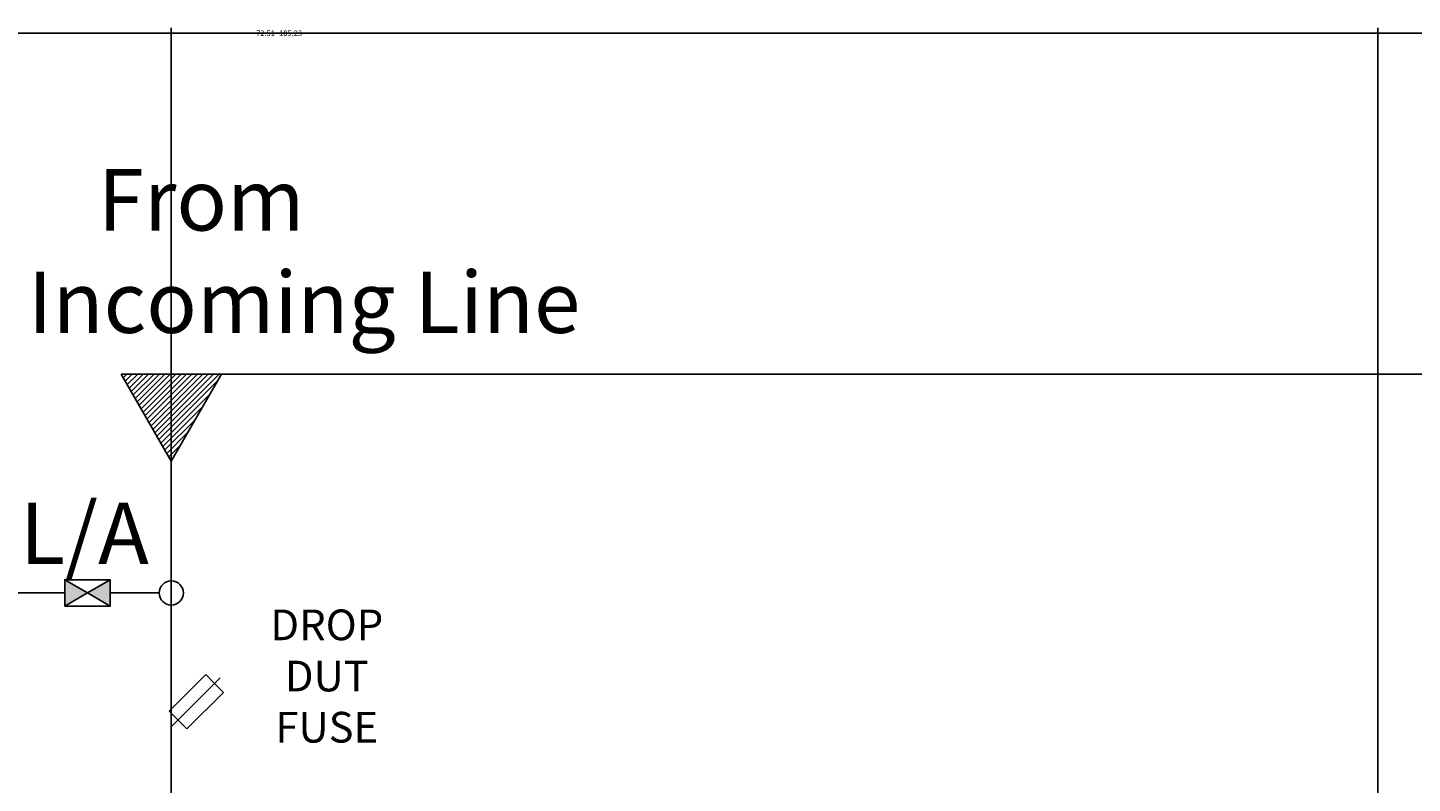
# Model space of a CAD drawing. Units: inches. Extents: x 412 to 584, y 208 to 437.
# Tile 27 of 28: x 495 to 540, y 413 to 437. Entities that reach past the tile are written whole.
import ezdxf

# ---------------------------------------------------------------- set-up
doc = ezdxf.new("R2010")
doc.units = ezdxf.units.IN
doc.header["$MEASUREMENT"] = 0
for name, color, linetype, lineweight in [('A-ANNO-DIMS', 2, 'Continuous', 18), ('E-ANNO-TEXT', 7, 'Continuous', 18), ('E-POWR-EQPM', 3, 'Continuous', 25), ('E-POWR-PATT', 3, 'Continuous', 13)]:
    doc.layers.add(name, color=color, linetype=linetype, lineweight=lineweight)
doc.styles.get("Standard").update_dxf_attribs({"font": 'arial.ttf'})
doc.dimstyles.get("Standard").update_dxf_attribs({"dimtxt": 0.18, "dimasz": 0.18, "dimexe": 0.18, "dimexo": 0.0625, "dimgap": 0.09, "dimtad": 0, "dimtih": 1, "dimtoh": 1, "dimdec": 4, "dimzin": 0, "dimdsep": 46, "dimtxsty": 'Standard', "dimcen": 0.09, "dimadec": 0, "dimazin": 0, "dimtfac": 1, "dimtdec": 4, "dimtofl": 0, "dimtmove": 0, "dimatfit": 3, "dimfxl": 1, "dimtolj": 1, "dimtzin": 0, "dimarcsym": 0})

# ---------------------------------------------------------------- blocks, each defined once
blk = doc.blocks.new('*D17')
at = {"layer": 'A-ANNO-DIMS', "color": 0, "lineweight": -2, "transparency": 16777216}
for p, q in [((497.715, 426.185), (583.674, 426.185)), ((583.494, 426.005), (583.494, 323.031)), ((583.494, 219.693), (583.494, 322.667)), ((550.198, 219.513), (583.674, 219.513))]:
    blk.add_line(p, q, dxfattribs=at)
at = {"layer": 'A-ANNO-DIMS', "color": 0, "transparency": 16777216}
for points in [[(583.464, 426.005), (583.524, 426.005), (583.494, 426.185)], [(583.464, 219.693), (583.524, 219.693), (583.494, 219.513)]]:
    blk.add_solid(points, dxfattribs=at)
at = {"layer": 'Defpoints', "color": 0, "transparency": 16777216}
for p in [(497.652, 426.185), (550.135, 219.513), (583.494, 219.513)]:
    blk.add_point(p, dxfattribs=at)
at = {"layer": 'A-ANNO-DIMS', "color": 0, "transparency": 16777216, "insert": (583.494, 322.849), "char_height": 0.18, "attachment_point": 5}
blk.add_mtext('\\A1;206.67', dxfattribs=at)
blk = doc.blocks.new('*D21')
at = {"layer": 'A-ANNO-DIMS', "color": 0, "lineweight": -2, "transparency": 16777216}
for p, q in [((466.104, 400.237), (466.104, 437.465)), ((538.619, 400.237), (538.619, 437.465)), ((466.284, 437.285), (501.986, 437.285)), ((538.439, 437.285), (502.737, 437.285))]:
    blk.add_line(p, q, dxfattribs=at)
at = {"layer": 'A-ANNO-DIMS', "color": 0, "transparency": 16777216}
for points in [[(466.284, 437.315), (466.284, 437.255), (466.104, 437.285)], [(538.439, 437.315), (538.439, 437.255), (538.619, 437.285)]]:
    blk.add_solid(points, dxfattribs=at)
at = {"layer": 'Defpoints', "color": 0, "transparency": 16777216}
for p in [(538.619, 437.285), (466.104, 400.175), (538.619, 400.175)]:
    blk.add_point(p, dxfattribs=at)
at = {"layer": 'A-ANNO-DIMS', "color": 0, "transparency": 16777216, "insert": (502.361, 437.285), "char_height": 0.18, "attachment_point": 5}
blk.add_mtext('\\A1;72.51', dxfattribs=at)
blk = doc.blocks.new('*D27')
at = {"layer": 'A-ANNO-DIMS', "color": 0, "lineweight": -2, "transparency": 16777216}
for p, q in [((466.104, 400.237), (466.104, 437.465)), ((499.288, 397.825), (499.288, 437.465)), ((466.284, 437.285), (482.233, 437.285)), ((499.108, 437.285), (483.159, 437.285))]:
    blk.add_line(p, q, dxfattribs=at)
at = {"layer": 'A-ANNO-DIMS', "color": 0, "transparency": 16777216}
for points in [[(466.284, 437.315), (466.284, 437.255), (466.104, 437.285)], [(499.108, 437.315), (499.108, 437.255), (499.288, 437.285)]]:
    blk.add_solid(points, dxfattribs=at)
at = {"layer": 'Defpoints', "color": 0, "transparency": 16777216}
for p in [(499.288, 437.285), (466.104, 400.175), (499.288, 397.763)]:
    blk.add_point(p, dxfattribs=at)
at = {"layer": 'A-ANNO-DIMS', "color": 0, "transparency": 16777216, "insert": (482.696, 437.285), "char_height": 0.18, "attachment_point": 5}
blk.add_mtext('\\A1;33.184', dxfattribs=at)
blk = doc.blocks.new('*D28')
at = {"layer": 'A-ANNO-DIMS', "color": 0, "lineweight": -2, "transparency": 16777216}
for p, q in [((450.562, 256.635), (450.562, 437.465)), ((555.796, 256.635), (555.796, 437.465)), ((450.742, 437.285), (502.724, 437.285)), ((555.616, 437.285), (503.634, 437.285))]:
    blk.add_line(p, q, dxfattribs=at)
at = {"layer": 'A-ANNO-DIMS', "color": 0, "transparency": 16777216}
for points in [[(450.742, 437.315), (450.742, 437.255), (450.562, 437.285)], [(555.616, 437.315), (555.616, 437.255), (555.796, 437.285)]]:
    blk.add_solid(points, dxfattribs=at)
at = {"layer": 'Defpoints', "color": 0, "transparency": 16777216}
for p in [(555.796, 437.285), (450.562, 256.573), (555.796, 256.573)]:
    blk.add_point(p, dxfattribs=at)
at = {"layer": 'A-ANNO-DIMS', "color": 0, "transparency": 16777216, "insert": (503.179, 437.285), "char_height": 0.18, "attachment_point": 5}
blk.add_mtext('\\A1;105.23', dxfattribs=at)

msp = doc.modelspace()

# ---------------------------------------------------------------- hatches: boundary and pattern name
at = {"layer": 'E-POWR-PATT'}
h = msp.add_hatch(dxfattribs=at)
h.set_pattern_fill('ANSI31', color=256)
h.set_pattern_definition([(45, (474.54576, 404.48029), (-0.08838835, 0.08838835), [])])
h.paths.add_polyline_path([(497.6523, 426.1847), (499.2878, 423.3518), (500.9234, 426.1847)])
h = msp.add_hatch(color=256, dxfattribs=at)
h.dxf.hatch_style = 1
h.paths.add_polyline_path([(495.8126, 419.4834), (495.8126, 418.6271), (496.5542, 419.0552)])
h.paths.add_polyline_path([(497.2958, 419.4834), (496.5542, 419.0552), (497.2958, 418.6271)])

# ---------------------------------------------------------------- linework, layer by layer
at = {"layer": 'E-POWR-EQPM'}
for p, q in [((499.2878, 423.3518), (499.2878, 419.4487)), ((495.8126, 419.0552), (494.1202, 419.0552)), ((498.8944, 419.0552), (497.2958, 419.0552)), ((499.2878, 418.6618), (499.2878, 416.2868)), ((499.2198, 415.2048), (500.4091, 416.3941)), ((499.2878, 414.6932), (500.8814, 416.2868)), ((500.4091, 416.3941), (500.6989, 416.1043)), ((499.7994, 414.6252), (500.9888, 415.8145)), ((500.9888, 415.8145), (500.6989, 416.1043)), ((499.5096, 414.915), (499.2198, 415.2048)), ((499.5096, 414.915), (499.7994, 414.6252)), ((499.2878, 414.6932), (499.2878, 411.7856))]:
    msp.add_line(p, q, dxfattribs=at)
for points in [[(497.6523, 426.1847), (499.2878, 423.3518), (500.9234, 426.1847)], [(496.5542, 419.0552), (495.8126, 418.6271), (495.8126, 419.4834)], [(495.8126, 419.4834), (497.2958, 419.4834), (497.2958, 418.6271), (495.8126, 418.6271)], [(496.5542, 419.0552), (497.2958, 418.6271), (497.2958, 419.4834)]]:
    msp.add_lwpolyline(points, close=True, dxfattribs=at)
msp.add_circle((499.2878, 419.0552), 0.3935, dxfattribs=at)

# ---------------------------------------------------------------- texts
at = {"layer": 'E-ANNO-TEXT', "attachment_point": 1}
for s, width, heights, insert, char_height in [('\\pxqc;From\\P11kV Incoming Line', 27.755796, [8.8771], (486.3843, 432.8579), 2), ('\\pxqc;L/A', 13.633448, [2.9648], (489.6366, 421.9937), 2), ('\\pxqc;DROP\\PDUT\\PFUSE\\P', 14.23487, [10.3993], (497.2401, 418.5147), 1)]:
    msp.add_mtext_dynamic_manual_height_columns(s, width=width, gutter_width=1, heights=heights, dxfattribs=dict(at, insert=insert, char_height=char_height))

# ---------------------------------------------------------------- dimensions: what is measured, and where the dimension line sits
at = {"layer": 'A-ANNO-DIMS'}
for base, p1, p2, override, picture, middle in [((555.7959, 437.2847), (450.562, 256.5729), (555.7959, 256.5729), {"dimdec": 2, "dimlfac": 1, "dimrnd": 0, "dimzin": 0, "dimdsep": 46, "dimlunit": 2}, '*D28', (503.1789, 437.2847)), ((538.6186, 437.2847), (466.1037, 400.175), (538.6186, 400.175), {"dimdec": 2, "dimlfac": 1, "dimrnd": 0, "dimzin": 0, "dimdsep": 46, "dimlunit": 2}, '*D21', (502.3612, 437.2847)), ((499.2878, 437.2847), (466.1037, 400.175), (499.2878, 397.7626), {"dimdec": 3, "dimlfac": 1, "dimrnd": 0, "dimzin": 0, "dimdsep": 46, "dimlunit": 2}, '*D27', (482.6958, 437.2847))]:
    dim = msp.add_linear_dim(base=base, p1=p1, p2=p2, dimstyle='Standard', override=override, dxfattribs=at)
    dim.commit()
    dim.dimension.update_dxf_attribs({"geometry": picture, "text_midpoint": middle})
dim = msp.add_linear_dim(base=(583.4937, 219.5133), p1=(497.6523, 426.1847), p2=(550.1351, 219.5133), angle=90, dimstyle='Standard', override={"dimdec": 2, "dimlfac": 1, "dimrnd": 0, "dimzin": 0, "dimdsep": 46, "dimlunit": 2}, dxfattribs=at)
dim.commit()
dim.dimension.update_dxf_attribs({"geometry": '*D17', "text_midpoint": (583.4937, 322.849)})

doc.saveas('drawing.dxf')
